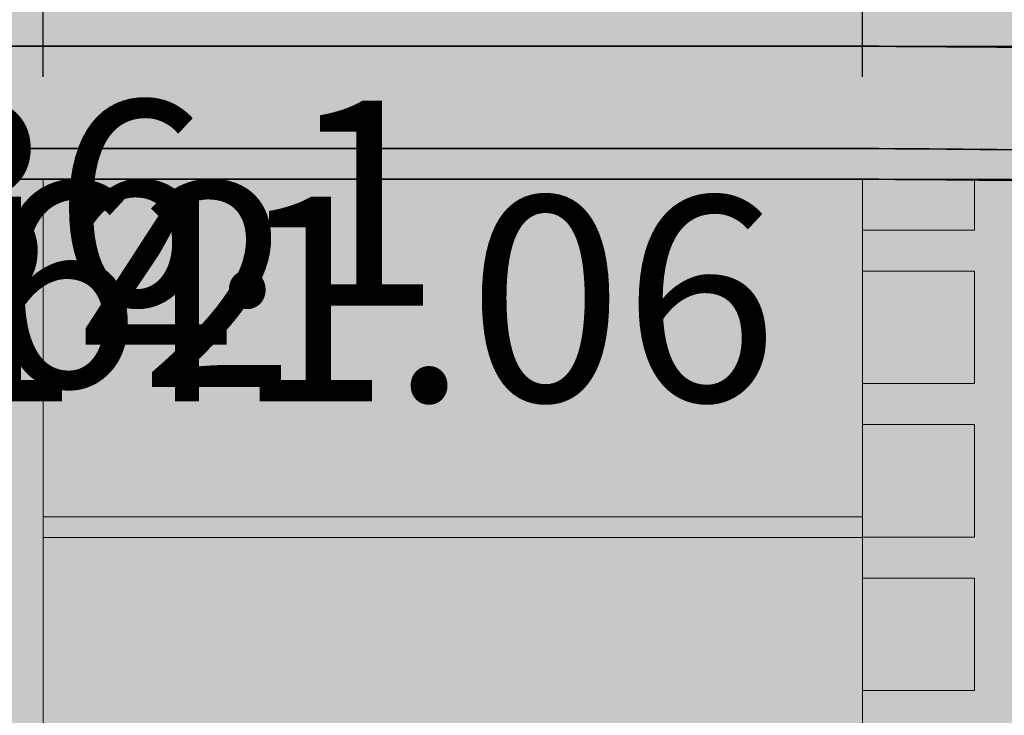
# Model space of a CAD drawing. Units: millimetres. Extents: x 130 to 1021, y 147 to 699.
# Tile 37 of 40: x 550 to 646, y 532 to 600. Entities that reach past the tile are written whole.
import ezdxf

# ---------------------------------------------------------------- set-up
doc = ezdxf.new("R2010")
doc.units = ezdxf.units.MM
doc.header["$MEASUREMENT"] = 0
for name, color, linetype, lineweight in [('A-ANNO-DIMS', 2, 'Continuous', 18), ('A-ELEV', 7, 'Continuous', 35), ('A-ELEV-PATT', 9, 'Continuous', 13), ('A-GLAZ', 4, 'Continuous', 18)]:
    doc.layers.add(name, color=color, linetype=linetype, lineweight=lineweight)
doc.styles.get("Standard").update_dxf_attribs({"font": 'arial.ttf'})
doc.dimstyles.get("Standard").update_dxf_attribs({"dimtxt": 20, "dimasz": 10, "dimexe": 10, "dimexo": 10, "dimgap": 5, "dimtad": 0, "dimtih": 1, "dimtoh": 1, "dimdec": 0, "dimzin": 0, "dimdsep": 46, "dimtxsty": 'Standard', "dimcen": 5, "dimadec": 0, "dimazin": 0, "dimtfac": 1, "dimtdec": 0, "dimtofl": 0, "dimtmove": 0, "dimatfit": 3, "dimfxl": 1, "dimtolj": 1, "dimtzin": 0, "dimarcsym": 0})

# ---------------------------------------------------------------- blocks, each defined once
blk = doc.blocks.new('*D11')
at = {"layer": 'A-ANNO-DIMS', "color": 0, "lineweight": -2, "transparency": 16777216}
for p, q in [((737.374, 648.699), (737.374, 149.739)), ((299.374, 566.947), (299.374, 149.739)), ((309.374, 159.739), (490.857, 159.739)), ((727.374, 159.739), (545.891, 159.739))]:
    blk.add_line(p, q, dxfattribs=at)
at = {"layer": 'A-ANNO-DIMS', "color": 0, "transparency": 16777216}
for points in [[(309.374, 161.406), (309.374, 158.073), (299.374, 159.739)], [(727.374, 161.406), (727.374, 158.073), (737.374, 159.739)]]:
    blk.add_solid(points, dxfattribs=at)
at = {"layer": 'Defpoints', "color": 0, "transparency": 16777216}
for p in [(737.374, 658.699), (299.374, 576.947), (737.374, 159.739)]:
    blk.add_point(p, dxfattribs=at)
at = {"layer": 'A-ANNO-DIMS', "color": 0, "transparency": 16777216, "insert": (518.374, 159.739), "char_height": 20, "attachment_point": 5}
blk.add_mtext('\\A1;438', dxfattribs=at)
blk = doc.blocks.new('*D22')
at = {"layer": 'A-ANNO-DIMS', "color": 0, "lineweight": -2, "transparency": 16777216}
for p, q in [((447.374, 656.947), (447.374, 696.247)), ((466.767, 403.947), (466.767, 696.247)), ((437.374, 686.247), (427.374, 686.247)), ((476.767, 686.247), (486.767, 686.247))]:
    blk.add_line(p, q, dxfattribs=at)
at = {"layer": 'A-ANNO-DIMS', "color": 0, "transparency": 16777216}
for points in [[(437.374, 687.914), (437.374, 684.581), (447.374, 686.247)], [(476.767, 687.914), (476.767, 684.581), (466.767, 686.247)]]:
    blk.add_solid(points, dxfattribs=at)
at = {"layer": 'Defpoints', "color": 0, "transparency": 16777216}
for p in [(466.767, 686.247), (447.374, 646.947), (466.767, 393.947)]:
    blk.add_point(p, dxfattribs=at)
at = {"layer": 'A-ANNO-DIMS', "color": 0, "transparency": 16777216, "insert": (532.34, 686.247), "char_height": 20, "attachment_point": 5}
blk.add_mtext('\\A1;19.393', dxfattribs=at)
blk = doc.blocks.new('*D23')
at = {"layer": 'A-ANNO-DIMS', "color": 0, "lineweight": -2, "transparency": 16777216}
for p, q in [((466.767, 403.947), (466.767, 696.247)), ((475.988, 209.039), (475.988, 696.247)), ((456.767, 686.247), (446.767, 686.247)), ((485.988, 686.247), (495.988, 686.247))]:
    blk.add_line(p, q, dxfattribs=at)
at = {"layer": 'A-ANNO-DIMS', "color": 0, "transparency": 16777216}
for points in [[(456.767, 687.914), (456.767, 684.581), (466.767, 686.247)], [(485.988, 687.914), (485.988, 684.581), (475.988, 686.247)]]:
    blk.add_solid(points, dxfattribs=at)
at = {"layer": 'Defpoints', "color": 0, "transparency": 16777216}
for p in [(475.988, 686.247), (466.767, 393.947), (475.988, 199.039)]:
    blk.add_point(p, dxfattribs=at)
at = {"layer": 'A-ANNO-DIMS', "color": 0, "transparency": 16777216, "insert": (534.631, 686.247), "char_height": 20, "attachment_point": 5}
blk.add_mtext('\\A1;9.222', dxfattribs=at)
blk = doc.blocks.new('*D24')
at = {"layer": 'A-ANNO-DIMS', "color": 0, "lineweight": -2, "transparency": 16777216}
for p, q in [((475.988, 209.039), (475.988, 696.247)), ((487.374, 671.947), (487.374, 696.247)), ((465.988, 686.247), (455.988, 686.247)), ((497.374, 686.247), (507.374, 686.247))]:
    blk.add_line(p, q, dxfattribs=at)
at = {"layer": 'A-ANNO-DIMS', "color": 0, "transparency": 16777216}
for points in [[(465.988, 687.914), (465.988, 684.581), (475.988, 686.247)], [(497.374, 687.914), (497.374, 684.581), (487.374, 686.247)]]:
    blk.add_solid(points, dxfattribs=at)
at = {"layer": 'Defpoints', "color": 0, "transparency": 16777216}
for p in [(487.374, 686.247), (487.374, 661.947), (475.988, 199.039)]:
    blk.add_point(p, dxfattribs=at)
at = {"layer": 'A-ANNO-DIMS', "color": 0, "transparency": 16777216, "insert": (553.022, 686.247), "char_height": 20, "attachment_point": 5}
blk.add_mtext('\\A1;11.385', dxfattribs=at)
blk = doc.blocks.new('*D25')
at = {"layer": 'A-ANNO-DIMS', "color": 0, "lineweight": -2, "transparency": 16777216}
for p, q in [((487.374, 671.947), (487.374, 696.247)), ((494.102, 506.908), (494.102, 696.247)), ((477.374, 686.247), (467.374, 686.247)), ((504.102, 686.247), (514.102, 686.247))]:
    blk.add_line(p, q, dxfattribs=at)
at = {"layer": 'A-ANNO-DIMS', "color": 0, "transparency": 16777216}
for points in [[(477.374, 687.914), (477.374, 684.581), (487.374, 686.247)], [(504.102, 687.914), (504.102, 684.581), (494.102, 686.247)]]:
    blk.add_solid(points, dxfattribs=at)
at = {"layer": 'Defpoints', "color": 0, "transparency": 16777216}
for p in [(494.102, 686.247), (487.374, 661.947), (494.102, 496.908)]:
    blk.add_point(p, dxfattribs=at)
at = {"layer": 'A-ANNO-DIMS', "color": 0, "transparency": 16777216, "insert": (552.922, 686.247), "char_height": 20, "attachment_point": 5}
blk.add_mtext('\\A1;6.728', dxfattribs=at)
blk = doc.blocks.new('*D26')
at = {"layer": 'A-ANNO-DIMS', "color": 0, "lineweight": -2, "transparency": 16777216}
for p, q in [((494.102, 506.908), (494.102, 696.247)), ((502.374, 593.947), (502.374, 696.247)), ((484.102, 686.247), (474.102, 686.247)), ((512.374, 686.247), (522.374, 686.247))]:
    blk.add_line(p, q, dxfattribs=at)
at = {"layer": 'A-ANNO-DIMS', "color": 0, "transparency": 16777216}
for points in [[(484.102, 687.914), (484.102, 684.581), (494.102, 686.247)], [(512.374, 687.914), (512.374, 684.581), (502.374, 686.247)]]:
    blk.add_solid(points, dxfattribs=at)
at = {"layer": 'Defpoints', "color": 0, "transparency": 16777216}
for p in [(502.374, 686.247), (502.374, 583.947), (494.102, 496.908)]:
    blk.add_point(p, dxfattribs=at)
at = {"layer": 'A-ANNO-DIMS', "color": 0, "transparency": 16777216, "insert": (561.03, 686.247), "char_height": 20, "attachment_point": 5}
blk.add_mtext('\\A1;8.272', dxfattribs=at)
blk = doc.blocks.new('*D27')
at = {"layer": 'A-ANNO-DIMS', "color": 0, "lineweight": -2, "transparency": 16777216}
for p, q in [((502.374, 593.947), (502.374, 696.247)), ((544.635, 396.264), (544.635, 696.247)), ((512.374, 686.247), (534.635, 686.247)), ((544.635, 686.247), (554.635, 686.247))]:
    blk.add_line(p, q, dxfattribs=at)
at = {"layer": 'A-ANNO-DIMS', "color": 0, "transparency": 16777216}
for points in [[(512.374, 687.914), (512.374, 684.581), (502.374, 686.247)], [(534.635, 687.914), (534.635, 684.581), (544.635, 686.247)]]:
    blk.add_solid(points, dxfattribs=at)
at = {"layer": 'Defpoints', "color": 0, "transparency": 16777216}
for p in [(544.635, 686.247), (502.374, 583.947), (544.635, 386.264)]:
    blk.add_point(p, dxfattribs=at)
at = {"layer": 'A-ANNO-DIMS', "color": 0, "transparency": 16777216, "insert": (593.776, 686.247), "char_height": 20, "attachment_point": 5}
blk.add_mtext('\\A1;42.26', dxfattribs=at)
blk = doc.blocks.new('*D28')
at = {"layer": 'A-ANNO-DIMS', "color": 0, "lineweight": -2, "transparency": 16777216}
for p, q in [((544.635, 396.264), (544.635, 696.247)), ((552.374, 593.947), (552.374, 696.247)), ((534.635, 686.247), (524.635, 686.247)), ((562.374, 686.247), (572.374, 686.247))]:
    blk.add_line(p, q, dxfattribs=at)
at = {"layer": 'A-ANNO-DIMS', "color": 0, "transparency": 16777216}
for points in [[(534.635, 687.914), (534.635, 684.581), (544.635, 686.247)], [(562.374, 687.914), (562.374, 684.581), (552.374, 686.247)]]:
    blk.add_solid(points, dxfattribs=at)
at = {"layer": 'Defpoints', "color": 0, "transparency": 16777216}
for p in [(552.374, 686.247), (552.374, 583.947), (544.635, 386.264)]:
    blk.add_point(p, dxfattribs=at)
at = {"layer": 'A-ANNO-DIMS', "color": 0, "transparency": 16777216, "insert": (611.057, 686.247), "char_height": 20, "attachment_point": 5}
blk.add_mtext('\\A1;7.738', dxfattribs=at)
blk = doc.blocks.new('*D29')
at = {"layer": 'A-ANNO-DIMS', "color": 0, "lineweight": -2, "transparency": 16777216}
for p, q in [((552.374, 593.947), (552.374, 696.247)), ((632.374, 593.947), (632.374, 696.247)), ((562.374, 686.247), (573.07, 686.247)), ((622.374, 686.247), (611.678, 686.247))]:
    blk.add_line(p, q, dxfattribs=at)
at = {"layer": 'A-ANNO-DIMS', "color": 0, "transparency": 16777216}
for points in [[(562.374, 687.914), (562.374, 684.581), (552.374, 686.247)], [(622.374, 687.914), (622.374, 684.581), (632.374, 686.247)]]:
    blk.add_solid(points, dxfattribs=at)
at = {"layer": 'Defpoints', "color": 0, "transparency": 16777216}
for p in [(632.374, 686.247), (552.374, 583.947), (632.374, 583.947)]:
    blk.add_point(p, dxfattribs=at)
at = {"layer": 'A-ANNO-DIMS', "color": 0, "transparency": 16777216, "insert": (592.374, 686.247), "char_height": 20, "attachment_point": 5}
blk.add_mtext('\\A1;80', dxfattribs=at)
blk = doc.blocks.new('*D30')
at = {"layer": 'A-ANNO-DIMS', "color": 0, "lineweight": -2, "transparency": 16777216}
for p, q in [((632.374, 593.947), (632.374, 696.247)), ((647.339, 584.979), (647.339, 696.247)), ((622.374, 686.247), (612.374, 686.247)), ((657.339, 686.247), (667.339, 686.247))]:
    blk.add_line(p, q, dxfattribs=at)
at = {"layer": 'A-ANNO-DIMS', "color": 0, "transparency": 16777216}
for points in [[(622.374, 687.914), (622.374, 684.581), (632.374, 686.247)], [(657.339, 687.914), (657.339, 684.581), (647.339, 686.247)]]:
    blk.add_solid(points, dxfattribs=at)
at = {"layer": 'Defpoints', "color": 0, "transparency": 16777216}
for p in [(647.339, 686.247), (632.374, 583.947), (647.339, 574.979)]:
    blk.add_point(p, dxfattribs=at)
at = {"layer": 'A-ANNO-DIMS', "color": 0, "transparency": 16777216, "insert": (712.987, 686.247), "char_height": 20, "attachment_point": 5}
blk.add_mtext('\\A1;14.965', dxfattribs=at)
blk = doc.blocks.new('*D31')
at = {"layer": 'A-ANNO-DIMS', "color": 0, "lineweight": -2, "transparency": 16777216}
for p, q in [((647.339, 584.979), (647.339, 696.247)), ((732.374, 653.96), (732.374, 696.247)), ((637.339, 686.247), (627.339, 686.247)), ((742.374, 686.247), (752.374, 686.247))]:
    blk.add_line(p, q, dxfattribs=at)
at = {"layer": 'A-ANNO-DIMS', "color": 0, "transparency": 16777216}
for points in [[(637.339, 687.914), (637.339, 684.581), (647.339, 686.247)], [(742.374, 687.914), (742.374, 684.581), (732.374, 686.247)]]:
    blk.add_solid(points, dxfattribs=at)
at = {"layer": 'Defpoints', "color": 0, "transparency": 16777216}
for p in [(732.374, 686.247), (732.374, 643.96), (647.339, 574.979)]:
    blk.add_point(p, dxfattribs=at)
at = {"layer": 'A-ANNO-DIMS', "color": 0, "transparency": 16777216, "insert": (689.857, 686.247), "char_height": 20, "attachment_point": 5}
blk.add_mtext('\\A1;85.03', dxfattribs=at)
blk = doc.blocks.new('*D56')
at = {"layer": 'A-ANNO-DIMS', "color": 0, "lineweight": -2, "transparency": 16777216}
for p, q in [((562.374, 583.947), (771.674, 583.947)), ((761.674, 573.947), (761.674, 545.659)), ((761.674, 486.947), (761.674, 515.236)), ((562.374, 476.947), (771.674, 476.947))]:
    blk.add_line(p, q, dxfattribs=at)
at = {"layer": 'A-ANNO-DIMS', "color": 0, "transparency": 16777216}
for points in [[(760.007, 573.947), (763.34, 573.947), (761.674, 583.947)], [(760.007, 486.947), (763.34, 486.947), (761.674, 476.947)]]:
    blk.add_solid(points, dxfattribs=at)
at = {"layer": 'Defpoints', "color": 0, "transparency": 16777216}
for p in [(552.374, 583.947), (761.674, 583.947), (552.374, 476.947)]:
    blk.add_point(p, dxfattribs=at)
at = {"layer": 'A-ANNO-DIMS', "color": 0, "transparency": 16777216, "insert": (761.674, 530.447), "char_height": 20, "attachment_point": 5}
blk.add_mtext('\\A1;107', dxfattribs=at)
blk = doc.blocks.new('*D57')
at = {"layer": 'A-ANNO-DIMS', "color": 0, "lineweight": -2, "transparency": 16777216}
for p, q in [((761.674, 606.947), (761.674, 616.947)), ((761.674, 616.947), (771.674, 616.947)), ((497.374, 596.947), (771.674, 596.947)), ((562.374, 583.947), (771.674, 583.947)), ((761.674, 573.947), (761.674, 563.947))]:
    blk.add_line(p, q, dxfattribs=at)
at = {"layer": 'A-ANNO-DIMS', "color": 0, "transparency": 16777216}
for points in [[(760.007, 606.947), (763.34, 606.947), (761.674, 596.947)], [(760.007, 573.947), (763.34, 573.947), (761.674, 583.947)]]:
    blk.add_solid(points, dxfattribs=at)
at = {"layer": 'Defpoints', "color": 0, "transparency": 16777216}
for p in [(487.374, 596.947), (761.674, 596.947), (552.374, 583.947)]:
    blk.add_point(p, dxfattribs=at)
at = {"layer": 'A-ANNO-DIMS', "color": 0, "transparency": 16777216, "insert": (790.057, 616.947), "char_height": 20, "attachment_point": 5}
blk.add_mtext('\\A1;13', dxfattribs=at)
blk = doc.blocks.new('*D58')
at = {"layer": 'A-ANNO-DIMS', "color": 0, "lineweight": -2, "transparency": 16777216}
for p, q in [((761.674, 656.947), (761.674, 666.947)), ((497.374, 646.947), (771.674, 646.947)), ((497.374, 596.947), (771.674, 596.947)), ((761.674, 586.947), (761.674, 576.947))]:
    blk.add_line(p, q, dxfattribs=at)
at = {"layer": 'A-ANNO-DIMS', "color": 0, "transparency": 16777216}
for points in [[(760.007, 656.947), (763.34, 656.947), (761.674, 646.947)], [(760.007, 586.947), (763.34, 586.947), (761.674, 596.947)]]:
    blk.add_solid(points, dxfattribs=at)
at = {"layer": 'Defpoints', "color": 0, "transparency": 16777216}
for p in [(487.374, 646.947), (761.674, 646.947), (487.374, 596.947)]:
    blk.add_point(p, dxfattribs=at)
at = {"layer": 'A-ANNO-DIMS', "color": 0, "transparency": 16777216, "insert": (761.674, 621.947), "char_height": 20, "attachment_point": 5}
blk.add_mtext('\\A1;50', dxfattribs=at)
blk = doc.blocks.new('*D69')
at = {"layer": 'A-ANNO-DIMS', "color": 0, "lineweight": -2, "transparency": 16777216}
for p, q in [((507.746, 572.261), (483.091, 501.813)), ((517.746, 572.261), (507.746, 572.261)), ((433.191, 354.23), (433.191, 364.23)), ((428.191, 359.23), (438.191, 359.23))]:
    blk.add_line(p, q, dxfattribs=at)
at = {"layer": 'A-ANNO-DIMS', "color": 0, "transparency": 16777216}
blk.add_solid([(481.518, 502.363), (484.664, 501.262), (479.788, 492.374)], dxfattribs=at)
at = {"layer": 'Defpoints', "color": 0, "transparency": 16777216}
for p in [(479.788, 492.374), (433.191, 359.23)]:
    blk.add_point(p, dxfattribs=at)
at = {"layer": 'A-ANNO-DIMS', "color": 0, "transparency": 16777216, "insert": (573.824, 572.261), "char_height": 20, "attachment_point": 5}
blk.add_mtext('\\A1;R141.06', dxfattribs=at)
blk = doc.blocks.new('*D71')
at = {"layer": 'A-ANNO-DIMS', "color": 0, "lineweight": -2, "transparency": 16777216}
for p, q in [((492.108, 581.609), (472.542, 512.666)), ((502.108, 581.609), (492.108, 581.609)), ((432.65, 367.109), (432.65, 377.109)), ((427.65, 372.109), (437.65, 372.109))]:
    blk.add_line(p, q, dxfattribs=at)
at = {"layer": 'A-ANNO-DIMS', "color": 0, "transparency": 16777216}
blk.add_solid([(470.938, 513.121), (474.145, 512.211), (469.812, 503.046)], dxfattribs=at)
at = {"layer": 'Defpoints', "color": 0, "transparency": 16777216}
for p in [(469.812, 503.046), (432.65, 372.109)]:
    blk.add_point(p, dxfattribs=at)
at = {"layer": 'A-ANNO-DIMS', "color": 0, "transparency": 16777216, "insert": (548.493, 581.609), "char_height": 20, "attachment_point": 5}
blk.add_mtext('\\A1;R136.1', dxfattribs=at)
blk = doc.blocks.new('*D72')
at = {"layer": 'A-ANNO-DIMS', "color": 0, "lineweight": -2, "transparency": 16777216}
for p, q in [((460.658, 573.64), (451.279, 503.49)), ((470.658, 573.64), (460.658, 573.64)), ((432.115, 355.142), (432.115, 365.142)), ((427.115, 360.142), (437.115, 360.142))]:
    blk.add_line(p, q, dxfattribs=at)
at = {"layer": 'A-ANNO-DIMS', "color": 0, "transparency": 16777216}
blk.add_solid([(449.628, 503.711), (452.931, 503.27), (449.954, 493.579)], dxfattribs=at)
at = {"layer": 'Defpoints', "color": 0, "transparency": 16777216}
for p in [(449.954, 493.579), (432.115, 360.142)]:
    blk.add_point(p, dxfattribs=at)
at = {"layer": 'A-ANNO-DIMS', "color": 0, "transparency": 16777216, "insert": (526.64, 573.64), "char_height": 20, "attachment_point": 5}
blk.add_mtext('\\A1;R134.62', dxfattribs=at)

msp = doc.modelspace()

# ---------------------------------------------------------------- hatches: boundary and pattern name
at = {"layer": 'A-ELEV-PATT'}
h = msp.add_hatch(color=256, dxfattribs=at)
h.dxf.hatch_style = 1
h.paths.add_polyline_path([(737.3738, 658.6988, 0.0135961), (632.4019, 661.9473), (607.3738, 661.9473), (487.3738, 661.9473), (487.3738, 649.9473), (607.3738, 649.9473), (632.3794, 649.9473, -0.0136841), (737.3738, 646.6784)])
h.paths.add_polyline_path([(732.3738, 643.9599, 0.0130529), (632.3738, 646.9473), (607.3738, 646.9473), (487.3738, 646.9473), (487.3738, 596.9473), (632.3738, 596.9473, -0.0130529), (732.3738, 593.9599)])
h.paths.add_polyline_path([(737.3738, 593.6732, 0.0137063), (632.3738, 596.9473), (487.3738, 596.9473), (487.3738, 586.9473), (632.355, 586.9473, -0.0137808), (737.3738, 583.6559)])
h.paths.add_polyline_path([(447.3738, 646.9473), (307.3738, 646.9473), (302.3738, 646.9473), (302.3738, 634.9473), (447.3738, 634.9473)])
h.paths.add_polyline_path([(447.3738, 631.9473), (307.3738, 631.9473), (307.3738, 586.9473), (447.3738, 586.9473)])
h.paths.add_polyline_path([(447.3738, 586.9473), (307.3738, 586.9473), (302.3738, 586.9473), (302.3738, 576.9473), (447.3738, 576.9473)])
h.paths.add_polyline_path([(447.3738, 573.9473), (367.3738, 573.9473), (367.3738, 539.9473), (447.3738, 539.9473)])
h.paths.add_polyline_path([(447.3738, 537.9473), (367.3738, 537.9473), (367.3738, 507.9473), (400.392, 507.4253, -0.001728), (401.3281, 507.6451, -0.5220025), (425.6117, 511.0391, -0.0391849), (447.3738, 510.4359), (447.3738, 510.7883)])
h.paths.add_polyline_path([(394.7238, 505.9473), (367.3738, 505.9473), (367.3738, 476.9473, -0.0146512), (375.8501, 480.2159), (376.1506, 499.2266, -0.0355419)])
h.paths.add_polyline_path([(632.3738, 583.9473), (552.3738, 583.9473), (552.3738, 550.9473), (632.3738, 550.9473)])
h.paths.add_polyline_path([(632.3738, 548.9473), (552.3738, 548.9473), (552.3738, 515.9473), (632.3738, 515.9473)])
h.paths.add_polyline_path([(632.3738, 513.9473), (552.3738, 513.9473), (552.3738, 476.9473), (632.3738, 476.9473)])
h.paths.add_polyline_path([(737.3738, 473.6903, 0.0136326), (632.3926, 476.9473), (552.3738, 476.9473), (487.3738, 476.9473), (487.3738, 466.9473), (632.3738, 466.9473, -0.0137063), (737.3738, 463.6732)])
h.paths.add_polyline_path([(732.3738, 460.9552, 0.0130741), (632.3681, 463.9473), (487.3738, 463.9473), (487.3738, 407.735, -0.0032286), (489.3544, 406.9473), (632.3926, 406.9473, -0.0129826), (732.3738, 403.9755)])
h.paths.add_polyline_path([(487.3738, 463.9473, 0.20133), (367.3738, 463.9473), (367.3738, 407.735, -0.1882031), (487.3738, 407.735)])
h.paths.add_polyline_path([(367.3738, 476.9473), (367.3738, 466.9473, -0.2013309), (487.3738, 466.9473), (487.3738, 476.9473, 0.20133)])
h.paths.add_polyline_path([(367.3738, 463.9473), (307.3738, 463.9473), (307.3738, 401.9473), (357.9413, 401.9473), (367.3738, 407.735)])
h.paths.add_polyline_path([(367.3738, 476.9473), (302.3738, 476.9473), (302.3738, 466.9473), (367.3738, 466.9473)])
h.paths.add_polyline_path([(632.8184, 366.9453), (552.3738, 366.9453), (552.3738, 393.9473), (632.8184, 393.9473)])
h.paths.add_polyline_path([(632.8184, 357.2114), (632.8184, 363.9453), (552.3738, 363.9453), (552.3738, 357.2114), (552.3738, 336.9453), (632.8184, 336.9453)])
h.paths.add_polyline_path([(632.8184, 333.9453), (552.3738, 333.9453), (552.3738, 306.9453), (632.8184, 306.9453)])
h.paths.add_polyline_path([(632.8184, 303.9453), (552.3738, 303.9453), (552.3738, 273.9473), (632.355, 273.9473, 0.0000608), (632.8184, 273.9491)])
h.paths.add_polyline_path([(737.3738, 403.6903, 0.0136326), (632.3926, 406.9473), (489.3544, 406.9473, 0.1915481), (367.3738, 407.735), (367.3738, 396.9473, -0.2013309), (487.3738, 396.9473), (632.3738, 396.9473, -0.0137063), (737.3738, 393.6732)])
h.paths.add_polyline_path([(357.9413, 401.9473), (307.3738, 401.9473), (307.3738, 391.9473), (357.9413, 391.9473)])
h.paths.add_polyline_path([(357.9413, 357.2114), (357.9413, 388.9473), (307.3738, 388.9473), (307.3738, 357.2114), (307.3738, 273.9473), (357.9413, 273.9473)])
h.paths.add_polyline_path([(732.3738, 263.93, -0.0130317), (632.3794, 260.9473), (466.7667, 260.9473), (466.7667, 240.9473), (469.8406, 236.978), (469.8406, 221.978), (472.9145, 218.0087), (472.9145, 213.9473), (607.3738, 213.9473), (732.3738, 213.9473)])
h.paths.add_polyline_path([(732.3738, 290.889), (722.479, 290.889), (722.479, 301.889), (732.3738, 301.889), (732.3738, 305.889), (722.479, 305.889), (722.479, 316.889), (732.3738, 316.889), (732.3738, 320.889), (722.479, 320.889), (722.479, 331.889), (732.3738, 331.889), (732.3738, 335.889), (722.479, 335.889), (722.479, 346.889), (732.3738, 346.889), (732.3738, 350.889), (722.479, 350.889), (722.479, 361.889), (732.3738, 361.889), (732.3738, 365.889), (722.479, 365.889), (722.479, 376.889), (732.3738, 376.889), (732.3738, 380.889), (722.479, 380.889), (722.479, 391.4848, 0.0005233), (718.479, 391.6843), (718.479, 380.889), (707.479, 380.889), (707.479, 392.1896, 0.0005231), (703.479, 392.3576), (703.479, 380.889), (692.479, 380.889), (692.479, 392.7765, 0.0005229), (688.479, 392.9131), (688.479, 380.889), (677.479, 380.889), (677.479, 393.2456, 0.0005228), (673.479, 393.3508), (673.479, 380.889), (662.479, 380.889), (662.479, 393.597, 0.0005227), (658.479, 393.6709), (658.479, 380.889), (647.479, 380.889), (647.479, 393.8308, 0.0005226), (643.479, 393.8732), (643.479, 380.889), (632.8184, 380.889), (632.8184, 376.889), (643.479, 376.889), (643.479, 365.889), (632.8184, 365.889), (632.8184, 361.889), (643.479, 361.889), (643.479, 350.889), (632.8184, 350.889), (632.8184, 346.889), (643.479, 346.889), (643.479, 335.889), (632.8184, 335.889), (632.8184, 331.889), (643.479, 331.889), (643.479, 320.889), (632.8184, 320.889), (632.8184, 316.889), (643.479, 316.889), (643.479, 305.889), (632.8184, 305.889), (632.8184, 301.889), (643.479, 301.889), (643.479, 290.889), (632.8184, 290.889), (632.8184, 286.889), (643.479, 286.889), (643.479, 274.0217, 0.0005246), (647.479, 274.0643), (647.479, 286.889), (658.479, 286.889), (658.479, 274.2248, 0.0005246), (662.479, 274.2989), (662.479, 286.889), (673.479, 286.889), (673.479, 274.546, 0.0005247), (677.479, 274.6516), (677.479, 286.889), (688.479, 286.889), (688.479, 274.9853, 0.0005248), (692.479, 275.1224), (692.479, 286.889), (703.479, 286.889), (703.479, 275.5429, 0.000525), (707.479, 275.7115), (707.479, 286.889), (718.479, 286.889), (718.479, 276.2187, 0.0005252), (722.479, 276.4189), (722.479, 286.889), (732.3738, 286.889)])
h.paths.add_polyline_path([(718.479, 290.889), (707.479, 290.889), (707.479, 301.889), (718.479, 301.889)], flags=16)
h.paths.add_polyline_path([(703.479, 290.889), (692.479, 290.889), (692.479, 301.889), (703.479, 301.889)], flags=16)
h.paths.add_polyline_path([(718.479, 305.889), (707.479, 305.889), (707.479, 316.889), (718.479, 316.889)], flags=16)
h.paths.add_polyline_path([(703.479, 305.889), (692.479, 305.889), (692.479, 316.889), (703.479, 316.889)], flags=16)
h.paths.add_polyline_path([(688.479, 290.889), (677.479, 290.889), (677.479, 301.889), (688.479, 301.889)], flags=16)
h.paths.add_polyline_path([(718.479, 320.889), (707.479, 320.889), (707.479, 331.889), (718.479, 331.889)], flags=16)
h.paths.add_polyline_path([(688.479, 305.889), (677.479, 305.889), (677.479, 316.889), (688.479, 316.889)], flags=16)
h.paths.add_polyline_path([(703.479, 320.889), (692.479, 320.889), (692.479, 331.889), (703.479, 331.889)], flags=16)
h.paths.add_polyline_path([(688.479, 320.889), (677.479, 320.889), (677.479, 331.889), (688.479, 331.889)], flags=16)
h.paths.add_polyline_path([(673.479, 290.889), (662.479, 290.889), (662.479, 301.889), (673.479, 301.889)], flags=16)
h.paths.add_polyline_path([(718.479, 335.889), (707.479, 335.889), (707.479, 346.889), (718.479, 346.889)], flags=16)
h.paths.add_polyline_path([(673.479, 305.889), (662.479, 305.889), (662.479, 316.889), (673.479, 316.889)], flags=16)
h.paths.add_polyline_path([(703.479, 335.889), (692.479, 335.889), (692.479, 346.889), (703.479, 346.889)], flags=16)
h.paths.add_polyline_path([(673.479, 320.889), (662.479, 320.889), (662.479, 331.889), (673.479, 331.889)], flags=16)
h.paths.add_polyline_path([(688.479, 335.889), (677.479, 335.889), (677.479, 346.889), (688.479, 346.889)], flags=16)
h.paths.add_polyline_path([(658.479, 290.889), (647.479, 290.889), (647.479, 301.889), (658.479, 301.889)], flags=16)
h.paths.add_polyline_path([(718.479, 350.889), (707.479, 350.889), (707.479, 361.889), (718.479, 361.889)], flags=16)
h.paths.add_polyline_path([(658.479, 305.889), (647.479, 305.889), (647.479, 316.889), (658.479, 316.889)], flags=16)
h.paths.add_polyline_path([(703.479, 350.889), (692.479, 350.889), (692.479, 361.889), (703.479, 361.889)], flags=16)
h.paths.add_polyline_path([(673.479, 335.889), (662.479, 335.889), (662.479, 346.889), (673.479, 346.889)], flags=16)
h.paths.add_polyline_path([(658.479, 320.889), (647.479, 320.889), (647.479, 331.889), (658.479, 331.889)], flags=16)
h.paths.add_polyline_path([(688.479, 350.889), (677.479, 350.889), (677.479, 361.889), (688.479, 361.889)], flags=16)
h.paths.add_polyline_path([(718.479, 365.889), (707.479, 365.889), (707.479, 376.889), (718.479, 376.889)], flags=16)
h.paths.add_polyline_path([(658.479, 335.889), (647.479, 335.889), (647.479, 346.889), (658.479, 346.889)], flags=16)
h.paths.add_polyline_path([(673.479, 350.889), (662.479, 350.889), (662.479, 361.889), (673.479, 361.889)], flags=16)
h.paths.add_polyline_path([(703.479, 365.889), (692.479, 365.889), (692.479, 376.889), (703.479, 376.889)], flags=16)
h.paths.add_polyline_path([(688.479, 365.889), (677.479, 365.889), (677.479, 376.889), (688.479, 376.889)], flags=16)
h.paths.add_polyline_path([(658.479, 350.889), (647.479, 350.889), (647.479, 361.889), (658.479, 361.889)], flags=16)
h.paths.add_polyline_path([(673.479, 365.889), (662.479, 365.889), (662.479, 376.889), (673.479, 376.889)], flags=16)
h.paths.add_polyline_path([(658.479, 365.889), (647.479, 365.889), (647.479, 376.889), (658.479, 376.889)], flags=16)
h.paths.add_polyline_path([(732.3738, 503.9786), (722.3392, 503.9786), (722.3392, 514.9786), (732.3738, 514.9786), (732.3738, 518.9786), (722.3392, 518.9786), (722.3392, 529.9786), (732.3738, 529.9786), (732.3738, 533.9786), (722.3392, 533.9786), (722.3392, 544.9786), (732.3738, 544.9786), (732.3738, 546.9473), (732.3738, 548.9786), (722.3392, 548.9786), (722.3392, 559.9786), (732.3738, 559.9786), (732.3738, 563.9786), (722.3392, 563.9786), (722.3392, 574.9786), (732.3738, 574.9786), (732.3738, 578.9786), (722.3392, 578.9786), (722.3392, 581.4789, 0.000526), (718.3392, 581.6791), (718.3392, 578.9786), (707.3392, 578.9786), (707.3392, 582.1863, 0.0005258), (703.3392, 582.355), (703.3392, 578.9786), (692.3392, 578.9786), (692.3392, 582.7752, 0.0005257), (688.3392, 582.9123), (688.3392, 578.9786), (677.3392, 578.9786), (677.3392, 583.2457, 0.0005255), (673.3392, 583.3512), (673.3392, 578.9786), (662.3392, 578.9786), (662.3392, 583.5978, 0.0005254), (658.3392, 583.6718), (658.3392, 578.9786), (647.3392, 578.9786), (647.3392, 583.8317, 0.0005254), (643.3392, 583.8741), (643.3392, 578.9786), (632.3738, 578.9786), (632.3738, 574.9786), (643.3392, 574.9786), (643.3392, 563.9786), (632.3738, 563.9786), (632.3738, 559.9786), (643.3392, 559.9786), (643.3392, 548.9786), (632.3738, 548.9786), (632.3738, 544.9786), (643.3392, 544.9786), (643.3392, 533.9786), (632.3738, 533.9786), (632.3738, 529.9786), (643.3392, 529.9786), (643.3392, 518.9786), (632.3738, 518.9786), (632.3738, 515.9473), (632.3738, 514.9786), (643.3392, 514.9786), (643.3392, 503.9786), (632.3738, 503.9786), (632.3738, 499.9786), (643.3392, 499.9786), (643.3392, 488.9786), (632.3738, 488.9786), (632.3738, 484.9786), (643.3392, 484.9786), (643.3392, 476.8751, -0.0005191), (647.3392, 476.8332), (647.3392, 484.9786), (658.3392, 484.9786), (658.3392, 476.6752, -0.0005192), (662.3392, 476.6022), (662.3392, 484.9786), (673.3392, 484.9786), (673.3392, 476.3585, -0.0005193), (677.3392, 476.2543), (677.3392, 484.9786), (688.3392, 484.9786), (688.3392, 475.9248, -0.0005194), (692.3392, 475.7894), (692.3392, 484.9786), (703.3392, 484.9786), (703.3392, 475.3741, -0.0005195), (707.3392, 475.2075), (707.3392, 484.9786), (718.3392, 484.9786), (718.3392, 474.7064, -0.0005197), (722.3392, 474.5086), (722.3392, 484.9786), (732.3738, 484.9786), (732.3738, 488.9786), (722.3392, 488.9786), (722.3392, 499.9786), (732.3738, 499.9786)])
h.paths.add_polyline_path([(718.3392, 503.9786), (707.3392, 503.9786), (707.3392, 514.9786), (718.3392, 514.9786)], flags=16)
h.paths.add_polyline_path([(718.3392, 499.9786), (718.3392, 488.9786), (707.3392, 488.9786), (707.3392, 499.9786)], flags=16)
h.paths.add_polyline_path([(718.3392, 518.9786), (707.3392, 518.9786), (707.3392, 529.9786), (718.3392, 529.9786)], flags=16)
h.paths.add_polyline_path([(703.3392, 503.9786), (692.3392, 503.9786), (692.3392, 514.9786), (703.3392, 514.9786)], flags=16)
h.paths.add_polyline_path([(703.3392, 499.9786), (703.3392, 488.9786), (692.3392, 488.9786), (692.3392, 499.9786)], flags=16)
h.paths.add_polyline_path([(703.3392, 518.9786), (692.3392, 518.9786), (692.3392, 529.9786), (703.3392, 529.9786)], flags=16)
h.paths.add_polyline_path([(718.3392, 533.9786), (707.3392, 533.9786), (707.3392, 544.9786), (718.3392, 544.9786)], flags=16)
h.paths.add_polyline_path([(688.3392, 503.9786), (677.3392, 503.9786), (677.3392, 514.9786), (688.3392, 514.9786)], flags=16)
h.paths.add_polyline_path([(688.3392, 499.9786), (688.3392, 488.9786), (677.3392, 488.9786), (677.3392, 499.9786)], flags=16)
h.paths.add_polyline_path([(703.3392, 533.9786), (692.3392, 533.9786), (692.3392, 544.9786), (703.3392, 544.9786)], flags=16)
h.paths.add_polyline_path([(688.3392, 518.9786), (677.3392, 518.9786), (677.3392, 529.9786), (688.3392, 529.9786)], flags=16)
h.paths.add_polyline_path([(688.3392, 533.9786), (677.3392, 533.9786), (677.3392, 544.9786), (688.3392, 544.9786)], flags=16)
h.paths.add_polyline_path([(718.3392, 548.9786), (707.3392, 548.9786), (707.3392, 559.9786), (718.3392, 559.9786)], flags=16)
h.paths.add_polyline_path([(673.3392, 503.9786), (662.3392, 503.9786), (662.3392, 514.9786), (673.3392, 514.9786)], flags=16)
h.paths.add_polyline_path([(673.3392, 499.9786), (673.3392, 488.9786), (662.3392, 488.9786), (662.3392, 499.9786)], flags=16)
h.paths.add_polyline_path([(703.3392, 548.9786), (692.3392, 548.9786), (692.3392, 559.9786), (703.3392, 559.9786)], flags=16)
h.paths.add_polyline_path([(673.3392, 518.9786), (662.3392, 518.9786), (662.3392, 529.9786), (673.3392, 529.9786)], flags=16)
h.paths.add_polyline_path([(688.3392, 548.9786), (677.3392, 548.9786), (677.3392, 559.9786), (688.3392, 559.9786)], flags=16)
h.paths.add_polyline_path([(673.3392, 533.9786), (662.3392, 533.9786), (662.3392, 544.9786), (673.3392, 544.9786)], flags=16)
h.paths.add_polyline_path([(718.3392, 563.9786), (707.3392, 563.9786), (707.3392, 574.9786), (718.3392, 574.9786)], flags=16)
h.paths.add_polyline_path([(658.3392, 503.9786), (647.3392, 503.9786), (647.3392, 514.9786), (658.3392, 514.9786)], flags=16)
h.paths.add_polyline_path([(658.3392, 499.9786), (658.3392, 488.9786), (647.3392, 488.9786), (647.3392, 499.9786)], flags=16)
h.paths.add_polyline_path([(703.3392, 563.9786), (692.3392, 563.9786), (692.3392, 574.9786), (703.3392, 574.9786)], flags=16)
h.paths.add_polyline_path([(658.3392, 518.9786), (647.3392, 518.9786), (647.3392, 529.9786), (658.3392, 529.9786)], flags=16)
h.paths.add_polyline_path([(673.3392, 548.9786), (662.3392, 548.9786), (662.3392, 559.9786), (673.3392, 559.9786)], flags=16)
h.paths.add_polyline_path([(688.3392, 563.9786), (677.3392, 563.9786), (677.3392, 574.9786), (688.3392, 574.9786)], flags=16)
h.paths.add_polyline_path([(658.3392, 533.9786), (647.3392, 533.9786), (647.3392, 544.9786), (658.3392, 544.9786)], flags=16)
h.paths.add_polyline_path([(673.3392, 563.9786), (662.3392, 563.9786), (662.3392, 574.9786), (673.3392, 574.9786)], flags=16)
h.paths.add_polyline_path([(658.3392, 548.9786), (647.3392, 548.9786), (647.3392, 559.9786), (658.3392, 559.9786)], flags=16)
h.paths.add_polyline_path([(658.3392, 563.9786), (647.3392, 563.9786), (647.3392, 574.9786), (658.3392, 574.9786)], flags=16)
h = msp.add_hatch(color=256, dxfattribs=at)
h.dxf.hatch_style = 1
h.paths.add_polyline_path([(447.3738, 576.9473), (302.3738, 576.9473), (302.3738, 573.9473), (447.3738, 573.9473)])
h.paths.add_polyline_path([(487.3738, 583.9473), (487.3738, 586.9473), (447.3738, 576.9473), (447.3738, 573.9473)])
h.paths.add_polyline_path([(632.355, 586.9473), (487.3738, 586.9473), (487.3738, 583.9473), (632.3738, 583.9473), (632.3738, 583.9472, -0.0138), (737.3738, 580.6507), (737.3738, 583.6559, 0.0137808)])
h.paths.add_polyline_path([(367.3738, 466.9473), (302.3738, 466.9473), (302.3738, 463.9473), (367.3738, 463.9473)])
h.paths.add_polyline_path([(487.3738, 463.9473), (487.3738, 466.9473, 0.2013309), (367.3738, 466.9473), (367.3738, 463.9473, -0.20133)])
h.paths.add_polyline_path([(632.3738, 466.9473), (487.3738, 466.9473), (487.3738, 463.9473), (632.3681, 463.9473, -0.0137285), (737.3738, 460.6681), (737.3738, 463.6732, 0.0137063)])
h.paths.add_polyline_path([(632.3738, 396.9473), (487.3738, 396.9473, 0.2013309), (367.3738, 396.9473), (367.3738, 393.9473, -0.2023717), (486.7667, 393.9473), (632.3681, 393.9473, -0.0137285), (737.3738, 390.6681), (737.3738, 393.6732, 0.0137063)])
h.paths.add_polyline_path([(357.9413, 391.9473), (307.3738, 391.9473), (307.3738, 388.9473), (357.9413, 388.9473)])
h.paths.add_polyline_path([(367.3738, 393.9473), (367.3738, 396.9473), (357.9413, 391.924), (357.9413, 388.9473), (358.058, 388.9473)])
h.paths.add_polyline_path([(737.3738, 264.2162), (737.3738, 267.2214, -0.0137063), (632.3738, 263.9473), (463.7667, 263.9473), (466.7667, 260.9473), (632.3794, 260.9473, 0.0136841)])
h.paths.add_polyline_path([(463.7667, 263.9473), (447.3738, 263.9473), (450.3738, 260.9473), (466.7667, 260.9473)])
h.paths.add_polyline_path([(447.3738, 263.9473), (432.3738, 263.9473), (432.3738, 260.9473), (450.3738, 260.9473)])
h.paths.add_polyline_path([(382.3738, 263.9473), (357.9413, 263.9473), (357.9413, 260.9473), (382.3738, 260.9473)])
h.paths.add_polyline_path([(357.9413, 263.9473), (307.3738, 263.9473), (307.3738, 260.9473), (357.9413, 260.9473)])
msp.add_hatch(color=256, dxfattribs=at).paths.add_polyline_path([(502.3738, 583.9473), (502.3738, 577.3739), (547.7773, 577.3739), (547.7773, 481.7432), (502.3738, 481.7432), (502.3738, 476.9473), (552.3738, 476.9473), (552.3738, 583.9473)])
h = msp.add_hatch(color=256, dxfattribs=at)
h.set_gradient(color1=(122, 175, 223), color2=(76, 153, 95))
h.paths.add_polyline_path([(632.3738, 484.9786), (632.3738, 476.9474, -0.001423), (643.3392, 476.8751), (643.3392, 484.9786)])
h.paths.add_polyline_path([(647.3392, 476.8332, -0.0014276), (658.3392, 476.6752), (658.3392, 484.9786), (647.3392, 484.9786)])
h.paths.add_polyline_path([(673.3392, 484.9786), (662.3392, 484.9786), (662.3392, 476.6022, -0.0014278), (673.3392, 476.3585)])
h.paths.add_polyline_path([(688.3392, 475.9248), (688.3392, 484.9786), (677.3392, 484.9786), (677.3392, 476.2543, -0.0014281)])
h.paths.add_polyline_path([(692.3392, 475.7894, -0.0014285), (703.3392, 475.3741), (703.3392, 484.9786), (692.3392, 484.9786)])
h.paths.add_polyline_path([(718.3392, 474.7064), (718.3392, 484.9786), (707.3392, 484.9786), (707.3392, 475.2075, -0.001429)])
h.paths.add_polyline_path([(722.3392, 474.5086, -0.001304), (732.3738, 473.9755), (732.3738, 484.9786), (722.3392, 484.9786)])
h.paths.add_polyline_path([(722.3392, 488.9786), (732.3738, 488.9786), (732.3738, 499.9786), (722.3392, 499.9786)])
h.paths.add_polyline_path([(707.3392, 499.9786), (707.3392, 488.9786), (718.3392, 488.9786), (718.3392, 499.9786)])
h.paths.add_polyline_path([(703.3392, 499.9786), (692.3392, 499.9786), (692.3392, 488.9786), (703.3392, 488.9786)])
h.paths.add_polyline_path([(688.3392, 499.9786), (677.3392, 499.9786), (677.3392, 488.9786), (688.3392, 488.9786)])
h.paths.add_polyline_path([(673.3392, 499.9786), (662.3392, 499.9786), (662.3392, 488.9786), (673.3392, 488.9786)])
h.paths.add_polyline_path([(658.3392, 499.9786), (647.3392, 499.9786), (647.3392, 488.9786), (658.3392, 488.9786)])
h.paths.add_polyline_path([(643.3392, 499.9786), (632.3738, 499.9786), (632.3738, 488.9786), (643.3392, 488.9786)])
h.paths.add_polyline_path([(643.3392, 514.9786), (632.3738, 514.9786), (632.3738, 503.9786), (643.3392, 503.9786)])
h.paths.add_polyline_path([(647.3392, 503.9786), (658.3392, 503.9786), (658.3392, 514.9786), (647.3392, 514.9786)])
h.paths.add_polyline_path([(673.3392, 514.9786), (662.3392, 514.9786), (662.3392, 503.9786), (673.3392, 503.9786)])
h.paths.add_polyline_path([(688.3392, 503.9786), (688.3392, 514.9786), (677.3392, 514.9786), (677.3392, 503.9786)])
h.paths.add_polyline_path([(692.3392, 503.9786), (703.3392, 503.9786), (703.3392, 514.9786), (692.3392, 514.9786)])
h.paths.add_polyline_path([(718.3392, 503.9786), (718.3392, 514.9786), (707.3392, 514.9786), (707.3392, 503.9786)])
h.paths.add_polyline_path([(732.3738, 503.9786), (732.3738, 514.9786), (722.3392, 514.9786), (722.3392, 503.9786)])
h.paths.add_polyline_path([(732.3738, 529.9786), (722.3392, 529.9786), (722.3392, 518.9786), (732.3738, 518.9786)])
h.paths.add_polyline_path([(707.3392, 518.9786), (718.3392, 518.9786), (718.3392, 529.9786), (707.3392, 529.9786)])
h.paths.add_polyline_path([(692.3392, 518.9786), (703.3392, 518.9786), (703.3392, 529.9786), (692.3392, 529.9786)])
h.paths.add_polyline_path([(688.3392, 529.9786), (677.3392, 529.9786), (677.3392, 518.9786), (688.3392, 518.9786)])
h.paths.add_polyline_path([(673.3392, 518.9786), (673.3392, 529.9786), (662.3392, 529.9786), (662.3392, 518.9786)])
h.paths.add_polyline_path([(658.3392, 529.9786), (647.3392, 529.9786), (647.3392, 518.9786), (658.3392, 518.9786)])
h.paths.add_polyline_path([(632.3738, 529.9786), (632.3738, 518.9786), (643.3392, 518.9786), (643.3392, 529.9786)])
h.paths.add_polyline_path([(643.3392, 533.9786), (643.3392, 544.9786), (632.3738, 544.9786), (632.3738, 533.9786)])
h.paths.add_polyline_path([(647.3392, 533.9786), (658.3392, 533.9786), (658.3392, 544.9786), (647.3392, 544.9786)])
h.paths.add_polyline_path([(662.3392, 533.9786), (673.3392, 533.9786), (673.3392, 544.9786), (662.3392, 544.9786)])
h.paths.add_polyline_path([(677.3392, 533.9786), (688.3392, 533.9786), (688.3392, 544.9786), (677.3392, 544.9786)])
h.paths.add_polyline_path([(692.3392, 533.9786), (703.3392, 533.9786), (703.3392, 544.9786), (692.3392, 544.9786)])
h.paths.add_polyline_path([(707.3392, 533.9786), (718.3392, 533.9786), (718.3392, 544.9786), (707.3392, 544.9786)])
h.paths.add_polyline_path([(722.3392, 533.9786), (732.3738, 533.9786), (732.3738, 544.9786), (722.3392, 544.9786)])
h.paths.add_polyline_path([(632.3738, 559.9786), (632.3738, 548.9786), (643.3392, 548.9786), (643.3392, 559.9786)])
h.paths.add_polyline_path([(632.3738, 574.9786), (632.3738, 563.9786), (643.3392, 563.9786), (643.3392, 574.9786)])
h.paths.add_polyline_path([(632.3738, 583.9472), (632.3738, 578.9786), (643.3392, 578.9786), (643.3392, 583.8741, 0.0014402)])
h.paths.add_polyline_path([(647.3392, 583.8317), (647.3392, 578.9786), (658.3392, 578.9786), (658.3392, 583.6718, 0.0014449)])
h.paths.add_polyline_path([(647.3392, 574.9786), (647.3392, 563.9786), (658.3392, 563.9786), (658.3392, 574.9786)])
h.paths.add_polyline_path([(647.3392, 559.9786), (647.3392, 548.9786), (658.3392, 548.9786), (658.3392, 559.9786)])
h.paths.add_polyline_path([(662.3392, 559.9786), (662.3392, 548.9786), (673.3392, 548.9786), (673.3392, 559.9786)])
h.paths.add_polyline_path([(673.3392, 574.9786), (662.3392, 574.9786), (662.3392, 563.9786), (673.3392, 563.9786)])
h.paths.add_polyline_path([(662.3392, 583.5978), (662.3392, 578.9786), (673.3392, 578.9786), (673.3392, 583.3512, 0.0014451)])
h.paths.add_polyline_path([(688.3392, 578.9786), (688.3392, 582.9123, 0.0014454), (677.3392, 583.2457), (677.3392, 578.9786)])
h.paths.add_polyline_path([(677.3392, 574.9786), (677.3392, 563.9786), (688.3392, 563.9786), (688.3392, 574.9786)])
h.paths.add_polyline_path([(677.3392, 559.9786), (677.3392, 548.9786), (688.3392, 548.9786), (688.3392, 559.9786)])
h.paths.add_polyline_path([(703.3392, 559.9786), (692.3392, 559.9786), (692.3392, 548.9786), (703.3392, 548.9786)])
h.paths.add_polyline_path([(707.3392, 548.9786), (718.3392, 548.9786), (718.3392, 559.9786), (707.3392, 559.9786)])
h.paths.add_polyline_path([(722.3392, 548.9786), (732.3738, 548.9786), (732.3738, 559.9786), (722.3392, 559.9786)])
h.paths.add_polyline_path([(732.3738, 563.9786), (732.3738, 574.9786), (722.3392, 574.9786), (722.3392, 563.9786)])
h.paths.add_polyline_path([(707.3392, 563.9786), (718.3392, 563.9786), (718.3392, 574.9786), (707.3392, 574.9786)])
h.paths.add_polyline_path([(692.3392, 563.9786), (703.3392, 563.9786), (703.3392, 574.9786), (692.3392, 574.9786)])
h.paths.add_polyline_path([(703.3392, 578.9786), (703.3392, 582.355, 0.0014458), (692.3392, 582.7752), (692.3392, 578.9786)])
h.paths.add_polyline_path([(718.3392, 581.6791, 0.0014463), (707.3392, 582.1863), (707.3392, 578.9786), (718.3392, 578.9786)])
h.paths.add_polyline_path([(732.3738, 578.9786), (732.3738, 580.9394, 0.0013198), (722.3392, 581.4789), (722.3392, 578.9786)])
h = msp.add_hatch(color=256, dxfattribs=at)
h.dxf.hatch_style = 1
h.paths.add_polyline_path([(447.3738, 537.9473), (447.3738, 539.9473), (367.3738, 539.9473), (367.3738, 537.9473)])
h.paths.add_polyline_path([(394.7238, 505.9473, -0.0105284), (400.392, 507.4253), (367.3738, 507.9473), (367.3738, 505.9473)])
h.paths.add_polyline_path([(547.7773, 546.9473), (547.7773, 548.9473), (502.3738, 548.9473), (502.3738, 546.9473)])
h.paths.add_polyline_path([(632.3738, 548.9473), (632.3738, 550.9473), (552.3738, 550.9473), (552.3738, 548.9473)])
h.paths.add_polyline_path([(632.3738, 513.9473), (632.3738, 515.9473), (552.3738, 515.9473), (552.3738, 513.9473)])
h.paths.add_polyline_path([(544.6354, 360.9453), (544.6354, 363.9453), (486.7667, 363.9454), (486.7667, 360.9454)])
h.paths.add_polyline_path([(632.8184, 363.9453), (632.8184, 366.9453), (552.3738, 366.9453), (552.3738, 363.9453)])
h.paths.add_polyline_path([(632.8184, 333.9453), (632.8184, 336.9453), (552.3738, 336.9453), (552.3738, 333.9453)])
h.paths.add_polyline_path([(552.3738, 306.9453), (552.3738, 303.9453), (632.8184, 303.9453), (632.8184, 306.9453)])

# ---------------------------------------------------------------- linework, layer by layer
at = {"layer": 'A-ELEV'}
for p, q in [((632.3738, 596.9473), (487.3738, 596.9473)), ((632.3738, 586.9473), (487.3738, 586.9473)), ((632.3738, 583.9473), (487.3738, 583.9473))]:
    msp.add_line(p, q, dxfattribs=at)
for radius, start in [(1916.4697, 86.6434721), (1906.4697, 86.6258458), (1903.4697, 86.6205218)]:
    msp.add_arc((625.1665, -1319.5089), radius, start, 89.784526, dxfattribs=at)
at = {"layer": 'A-GLAZ'}
for p, q in [((552.3738, 583.9473), (552.3738, 476.9473)), ((632.3738, 476.9473), (632.3738, 583.9473)), ((643.3392, 578.9786), (643.3392, 583.8741)), ((632.3738, 578.9786), (643.3392, 578.9786)), ((632.3738, 574.9786), (643.3392, 574.9786)), ((643.3392, 563.9786), (643.3392, 574.9786)), ((632.3738, 563.9786), (643.3392, 563.9786)), ((632.3738, 559.9786), (643.3392, 559.9786)), ((643.3392, 548.9786), (643.3392, 559.9786)), ((632.3738, 550.9473), (552.3738, 550.9473)), ((632.3738, 548.9473), (552.3738, 548.9473)), ((632.3738, 548.9786), (643.3392, 548.9786)), ((632.3738, 544.9786), (643.3392, 544.9786)), ((643.3392, 533.9786), (643.3392, 544.9786)), ((632.3738, 533.9786), (643.3392, 533.9786))]:
    msp.add_line(p, q, dxfattribs=at)

# ---------------------------------------------------------------- dimensions: what is measured, and where the dimension line sits
at = {"layer": 'A-ANNO-DIMS'}
for base, p1, p2, override, picture, middle in [((466.7667, 686.2473), (447.3738, 646.9473), (466.7667, 393.9473), {"dimdec": 3, "dimlfac": 1, "dimrnd": 0, "dimzin": 0, "dimdsep": 46, "dimlunit": 2}, '*D22', (532.3397, 686.2473)), ((475.9885, 686.2473), (466.7667, 393.9473), (475.9885, 199.0395), {"dimdec": 3, "dimlfac": 1, "dimrnd": 0, "dimzin": 0, "dimdsep": 46, "dimlunit": 2}, '*D23', (534.631, 686.2473)), ((487.3738, 686.2473), (475.9885, 199.0395), (487.3738, 661.9473), {"dimdec": 3, "dimlfac": 1, "dimrnd": 0, "dimzin": 0, "dimdsep": 46, "dimlunit": 2}, '*D24', (553.0218, 686.2473)), ((494.10227, 686.2473), (487.37378, 661.9473), (494.10227, 496.90803), {"dimdec": 3, "dimlfac": 1, "dimrnd": 0, "dimzin": 0, "dimdsep": 46, "dimlunit": 2}, '*D25', (552.92219, 686.2473)), ((502.37378, 686.2473), (494.10227, 496.90803), (502.37378, 583.9473), {"dimdec": 3, "dimlfac": 1, "dimrnd": 0, "dimzin": 0, "dimdsep": 46, "dimlunit": 2}, '*D26', (561.02999, 686.2473)), ((544.6354, 686.2473), (502.3738, 583.9473), (544.6354, 386.2639), {"dimdec": 2, "dimlfac": 1, "dimrnd": 0, "dimzin": 0, "dimdsep": 46, "dimlunit": 2}, '*D27', (593.776, 686.2473)), ((552.3738, 686.2473), (544.6354, 386.2639), (552.3738, 583.9473), {"dimdec": 3, "dimlfac": 1, "dimrnd": 0, "dimzin": 0, "dimdsep": 46, "dimlunit": 2}, '*D28', (611.0573, 686.2473)), ((632.3738, 686.2473), (552.3738, 583.9473), (632.3738, 583.9473), {"dimdec": 0, "dimlfac": 1, "dimrnd": 0, "dimzin": 0, "dimdsep": 46, "dimlunit": 2}, '*D29', (592.3738, 686.2473)), ((647.3392, 686.2473), (632.3738, 583.9473), (647.3392, 574.9786), {"dimdec": 3, "dimlfac": 1, "dimrnd": 0, "dimzin": 0, "dimdsep": 46, "dimlunit": 2}, '*D30', (712.9873, 686.2473)), ((732.3738, 686.2473), (647.3392, 574.9786), (732.3738, 643.9599), {"dimdec": 2, "dimlfac": 1, "dimrnd": 0, "dimzin": 0, "dimdsep": 46, "dimlunit": 2}, '*D31', (689.8565, 686.2473)), ((737.3738, 159.7395), (299.3738, 576.9473), (737.3738, 658.6988), {"dimdec": 0, "dimlfac": 1, "dimrnd": 0, "dimzin": 0, "dimdsep": 46, "dimlunit": 2}, '*D11', (518.3738, 159.7395))]:
    dim = msp.add_linear_dim(base=base, p1=p1, p2=p2, dimstyle='Standard', override=override, dxfattribs=at)
    dim.commit()
    dim.dimension.update_dxf_attribs({"geometry": picture, "text_midpoint": middle})
for base, p1, p2, picture, middle in [((761.6738, 646.9473), (487.3738, 596.9473), (487.3738, 646.9473), '*D58', (761.6738, 621.9473)), ((761.6738, 596.9473), (552.3738, 583.9473), (487.3738, 596.9473), '*D57', (790.0571, 616.9473)), ((761.6738, 583.9473), (552.3738, 476.9473), (552.3738, 583.9473), '*D56', (761.6738, 530.4473))]:
    dim = msp.add_linear_dim(base=base, p1=p1, p2=p2, angle=90, dimstyle='Standard', override={"dimdec": 0, "dimlfac": 1, "dimrnd": 0, "dimzin": 0, "dimdsep": 46, "dimlunit": 2}, dxfattribs=at)
    dim.commit()
    dim.dimension.update_dxf_attribs({"geometry": picture, "text_midpoint": middle})
for center, mpoint, override, picture, middle in [((432.6505, 372.1087), (469.8116, 503.0461), {"dimdec": 1, "dimlfac": 1, "dimrnd": 0, "dimzin": 0, "dimdsep": 46, "dimlunit": 2}, '*D71', (548.493, 581.6085)), ((432.115, 360.1423), (449.9544, 493.5786), {"dimdec": 2, "dimlfac": 1, "dimrnd": 0, "dimzin": 0, "dimdsep": 46, "dimlunit": 2}, '*D72', (526.6403, 573.6404)), ((433.1906, 359.2304), (479.788, 492.3743), {"dimdec": 2, "dimlfac": 1, "dimrnd": 0, "dimzin": 0, "dimdsep": 46, "dimlunit": 2}, '*D69', (573.8242, 572.2606))]:
    dim = msp.add_radius_dim(center=center, mpoint=mpoint, dimstyle='Standard', override=override, dxfattribs=at)
    dim.commit()
    dim.dimension.update_dxf_attribs({"geometry": picture, "text_midpoint": middle, "dimtype": 164})

doc.saveas('drawing.dxf')
